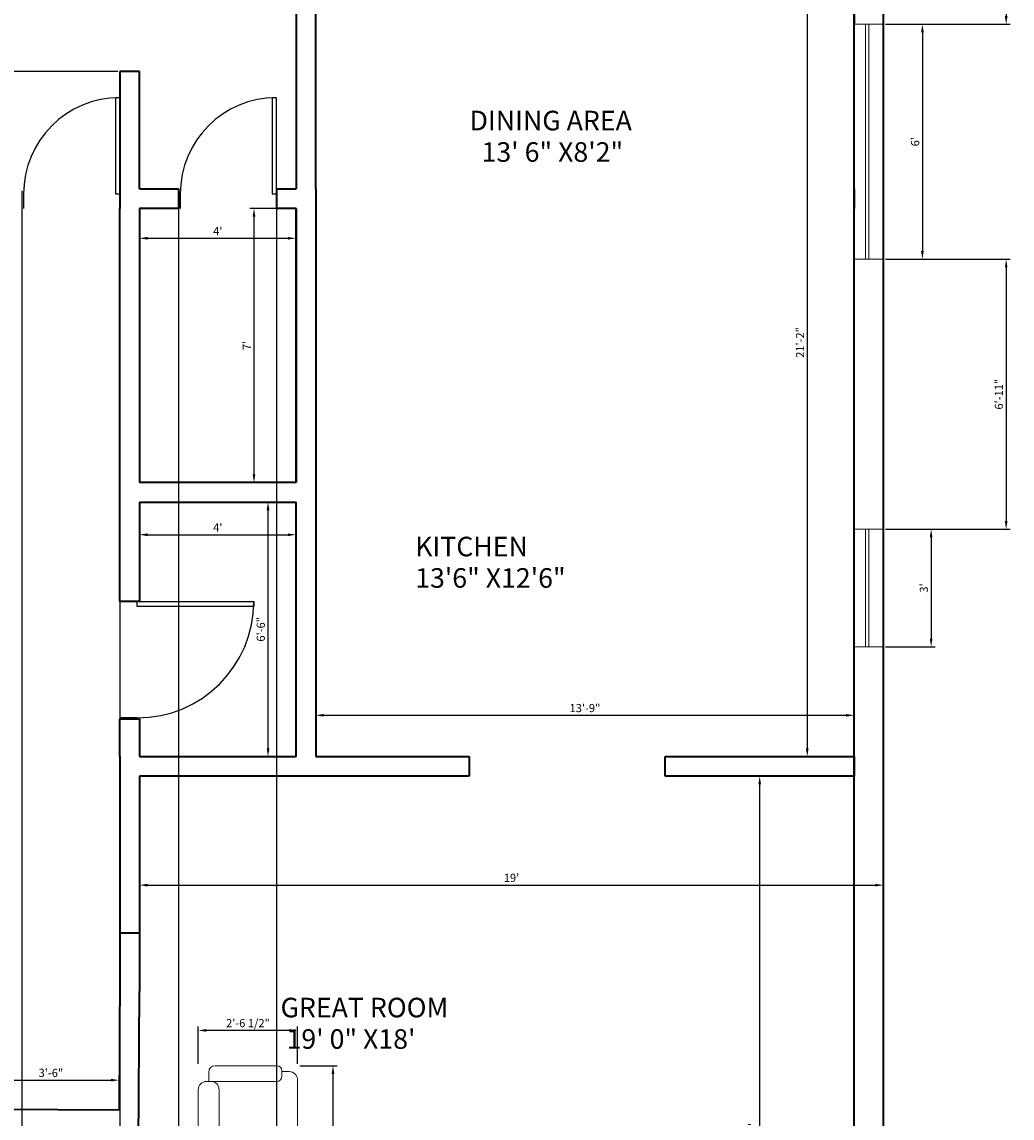
# Model space of a CAD drawing. Units: inches. Extents: x 2025 to 2528, y 1525 to 2336.
# Tile 8 of 18: x 2225 to 2528, y 1831 to 2167. Entities that reach past the tile are written whole.
import ezdxf

# ---------------------------------------------------------------- set-up
doc = ezdxf.new("R2010")
doc.units = ezdxf.units.IN
for name, color, linetype, lineweight in [('A-ANNO-DIMS', 2, 'Continuous', 18), ('A-AREA-IDEN', 7, 'Continuous', 25), ('A-DOOR', 3, 'Continuous', 25), ('A-FURN', 8, 'Continuous', 18), ('A-GLAZ', 4, 'Continuous', 18), ('A-WALL', 7, 'Continuous', 35)]:
    doc.layers.add(name, color=color, linetype=linetype, lineweight=lineweight)
doc.styles.get("Standard").update_dxf_attribs({"font": 'arial.ttf'})
doc.dimstyles.new('Copy of ISO-25', dxfattribs={"dimtxt": 2.5, "dimasz": 2.5, "dimexe": 1.25, "dimexo": 0.625, "dimtad": 1, "dimdec": 1, "dimlunit": 4, "dimtxsty": 'Standard', "dimcen": 2.5, "dimadec": 0, "dimazin": 0, "dimtfac": 1, "dimtdec": 1, "dimtmove": 0, "dimatfit": 3, "dimfxl": 1, "dimarcsym": 0})

# ---------------------------------------------------------------- blocks, each defined once
blk = doc.blocks.new('*U3')
for p, q in [((0, 0), (0, -6)), ((-40, 0), (-40, -6))]:
    blk.add_line(p, q)
blk.add_lwpolyline([(0, 0), (0, 40), (-1.75, 40), (-1.75, 0)], close=True)
blk.add_arc((0, 0), 40, 90, 180)
blk = doc.blocks.new('*U4')
for p, q in [((-40, 0), (-40, 6)), ((0, 0), (0, 6))]:
    blk.add_line(p, q)
blk.add_lwpolyline([(0, 0), (0, -40), (-1.75, -40), (-1.75, 0)], close=True)
blk.add_arc((0, 0), 40, 180, 270)
blk = doc.blocks.new('*D10')
at = {"layer": 'A-ANNO-DIMS', "color": 0, "lineweight": -2, "transparency": 16777216}
for p, q in [((2261.01, 2108.79), (2261.01, 2099)), ((2309.01, 2108.79), (2309.01, 2099)), ((2263.51, 2100.25), (2306.51, 2100.25))]:
    blk.add_line(p, q, dxfattribs=at)
at = {"layer": 'A-ANNO-DIMS', "color": 0, "transparency": 16777216}
for points in [[(2263.51, 2100.67), (2263.51, 2099.84), (2261.01, 2100.25)], [(2306.51, 2100.67), (2306.51, 2099.84), (2309.01, 2100.25)]]:
    blk.add_solid(points, dxfattribs=at)
at = {"layer": 'Defpoints', "color": 0, "transparency": 16777216}
for p in [(2261.01, 2109.41), (2309.01, 2109.41), (2309.01, 2100.25)]:
    blk.add_point(p, dxfattribs=at)
at = {"layer": 'A-ANNO-DIMS', "color": 0, "transparency": 16777216, "insert": (2285.01, 2102.13), "char_height": 2.5, "attachment_point": 5}
blk.add_mtext("4'", dxfattribs=at)
blk = doc.blocks.new('*D11')
at = {"layer": 'A-ANNO-DIMS', "color": 0, "lineweight": -2, "transparency": 16777216}
for p, q in [((2308.39, 2109.41), (2294.86, 2109.41)), ((2296.11, 2106.91), (2296.11, 2027.91)), ((2308.39, 2025.41), (2294.86, 2025.41))]:
    blk.add_line(p, q, dxfattribs=at)
at = {"layer": 'A-ANNO-DIMS', "color": 0, "transparency": 16777216}
for points in [[(2295.7, 2106.91), (2296.53, 2106.91), (2296.11, 2109.41)], [(2295.7, 2027.91), (2296.53, 2027.91), (2296.11, 2025.41)]]:
    blk.add_solid(points, dxfattribs=at)
at = {"layer": 'Defpoints', "color": 0, "transparency": 16777216}
for p in [(2309.01, 2109.41), (2296.11, 2025.41), (2309.01, 2025.41)]:
    blk.add_point(p, dxfattribs=at)
at = {"layer": 'A-ANNO-DIMS', "color": 0, "transparency": 16777216, "insert": (2294.24, 2067.41), "char_height": 2.5, "attachment_point": 5, "rotation": 90}
blk.add_mtext("7'", dxfattribs=at)
blk = doc.blocks.new('*D14')
at = {"layer": 'A-ANNO-DIMS', "color": 0, "lineweight": -2, "transparency": 16777216}
for p, q in [((2261.01, 2018.79), (2261.01, 2008.15)), ((2309.01, 2018.79), (2309.01, 2008.15)), ((2263.51, 2009.4), (2306.51, 2009.4))]:
    blk.add_line(p, q, dxfattribs=at)
at = {"layer": 'A-ANNO-DIMS', "color": 0, "transparency": 16777216}
for points in [[(2263.51, 2009.82), (2263.51, 2008.98), (2261.01, 2009.4)], [(2306.51, 2009.82), (2306.51, 2008.98), (2309.01, 2009.4)]]:
    blk.add_solid(points, dxfattribs=at)
at = {"layer": 'Defpoints', "color": 0, "transparency": 16777216}
for p in [(2261.01, 2019.41), (2309.01, 2019.41), (2309.01, 2009.4)]:
    blk.add_point(p, dxfattribs=at)
at = {"layer": 'A-ANNO-DIMS', "color": 0, "transparency": 16777216, "insert": (2285.01, 2011.27), "char_height": 2.5, "attachment_point": 5}
blk.add_mtext("4'", dxfattribs=at)
blk = doc.blocks.new('*D15')
at = {"layer": 'A-ANNO-DIMS', "color": 0, "lineweight": -2, "transparency": 16777216}
for p, q in [((2308.39, 2019.41), (2299.17, 2019.41)), ((2300.42, 1943.91), (2300.42, 2016.91)), ((2308.39, 1941.41), (2299.17, 1941.41))]:
    blk.add_line(p, q, dxfattribs=at)
at = {"layer": 'A-ANNO-DIMS', "color": 0, "transparency": 16777216}
for points in [[(2300.01, 2016.91), (2300.84, 2016.91), (2300.42, 2019.41)], [(2300.01, 1943.91), (2300.84, 1943.91), (2300.42, 1941.41)]]:
    blk.add_solid(points, dxfattribs=at)
at = {"layer": 'Defpoints', "color": 0, "transparency": 16777216}
for p in [(2300.42, 2019.41), (2309.01, 2019.41), (2309.01, 1941.41)]:
    blk.add_point(p, dxfattribs=at)
at = {"layer": 'A-ANNO-DIMS', "color": 0, "transparency": 16777216, "insert": (2298.52, 1980.41), "char_height": 2.5, "attachment_point": 5, "rotation": 90}
blk.add_mtext('6\'-6"', dxfattribs=at)
blk = doc.blocks.new('*D18')
at = {"layer": 'A-ANNO-DIMS', "color": 0, "lineweight": -2, "transparency": 16777216}
for p, q in [((2479.39, 2195.22), (2464.37, 2195.22)), ((2465.62, 2192.72), (2465.62, 1943.91)), ((2479.39, 1941.41), (2464.37, 1941.41))]:
    blk.add_line(p, q, dxfattribs=at)
at = {"layer": 'A-ANNO-DIMS', "color": 0, "transparency": 16777216}
for points in [[(2465.2, 2192.72), (2466.03, 2192.72), (2465.62, 2195.22)], [(2465.2, 1943.91), (2466.03, 1943.91), (2465.62, 1941.41)]]:
    blk.add_solid(points, dxfattribs=at)
at = {"layer": 'Defpoints', "color": 0, "transparency": 16777216}
for p in [(2480.01, 2195.22), (2465.62, 1941.41), (2480.01, 1941.41)]:
    blk.add_point(p, dxfattribs=at)
at = {"layer": 'A-ANNO-DIMS', "color": 0, "transparency": 16777216, "insert": (2463.74, 2068.31), "char_height": 2.5, "attachment_point": 5, "rotation": 90}
blk.add_mtext('21\'-2"', dxfattribs=at)
blk = doc.blocks.new('*D19')
at = {"layer": 'A-ANNO-DIMS', "color": 0, "lineweight": -2, "transparency": 16777216}
for p, q in [((2315.01, 1942.04), (2315.01, 1955.31)), ((2480.01, 1942.04), (2480.01, 1955.31)), ((2317.51, 1954.06), (2477.51, 1954.06))]:
    blk.add_line(p, q, dxfattribs=at)
at = {"layer": 'A-ANNO-DIMS', "color": 0, "transparency": 16777216}
for points in [[(2317.51, 1954.48), (2317.51, 1953.64), (2315.01, 1954.06)], [(2477.51, 1954.48), (2477.51, 1953.64), (2480.01, 1954.06)]]:
    blk.add_solid(points, dxfattribs=at)
at = {"layer": 'Defpoints', "color": 0, "transparency": 16777216}
for p in [(2480.01, 1954.06), (2315.01, 1941.41), (2480.01, 1941.41)]:
    blk.add_point(p, dxfattribs=at)
at = {"layer": 'A-ANNO-DIMS', "color": 0, "transparency": 16777216, "insert": (2397.51, 1955.96), "char_height": 2.5, "attachment_point": 5}
blk.add_mtext('13\'-9"', dxfattribs=at)
blk = doc.blocks.new('*D23')
at = {"layer": 'A-ANNO-DIMS', "color": 0, "lineweight": -2, "transparency": 16777216}
for p, q in [((2489.64, 2011.08), (2504.83, 2011.08)), ((2503.58, 2008.58), (2503.58, 1977.58)), ((2489.64, 1975.08), (2504.83, 1975.08))]:
    blk.add_line(p, q, dxfattribs=at)
at = {"layer": 'A-ANNO-DIMS', "color": 0, "transparency": 16777216}
for points in [[(2503.16, 2008.58), (2504, 2008.58), (2503.58, 2011.08)], [(2503.16, 1977.58), (2504, 1977.58), (2503.58, 1975.08)]]:
    blk.add_solid(points, dxfattribs=at)
at = {"layer": 'Defpoints', "color": 0, "transparency": 16777216}
for p in [(2489.01, 2011.08), (2489.01, 1975.08), (2503.58, 1975.08)]:
    blk.add_point(p, dxfattribs=at)
at = {"layer": 'A-ANNO-DIMS', "color": 0, "transparency": 16777216, "insert": (2501.68, 1993.08), "char_height": 2.5, "attachment_point": 5, "rotation": 90}
blk.add_mtext("3'", dxfattribs=at)
blk = doc.blocks.new('*D24')
at = {"layer": 'A-ANNO-DIMS', "color": 0, "lineweight": -2, "transparency": 16777216}
for p, q in [((2489.64, 2165.84), (2502.15, 2165.84)), ((2500.9, 2163.34), (2500.9, 2096.34)), ((2489.64, 2093.84), (2502.15, 2093.84))]:
    blk.add_line(p, q, dxfattribs=at)
at = {"layer": 'A-ANNO-DIMS', "color": 0, "transparency": 16777216}
for points in [[(2500.48, 2163.34), (2501.32, 2163.34), (2500.9, 2165.84)], [(2500.48, 2096.34), (2501.32, 2096.34), (2500.9, 2093.84)]]:
    blk.add_solid(points, dxfattribs=at)
at = {"layer": 'Defpoints', "color": 0, "transparency": 16777216}
for p in [(2489.01, 2165.84), (2489.01, 2093.84), (2500.9, 2093.84)]:
    blk.add_point(p, dxfattribs=at)
at = {"layer": 'A-ANNO-DIMS', "color": 0, "transparency": 16777216, "insert": (2499, 2129.84), "char_height": 2.5, "attachment_point": 5, "rotation": 90}
blk.add_mtext("6'", dxfattribs=at)
blk = doc.blocks.new('*D31')
at = {"layer": 'A-ANNO-DIMS', "color": 0, "lineweight": -2, "transparency": 16777216}
for p, q in [((2479.39, 1935.41), (2449.8, 1935.41)), ((2451.05, 1715.91), (2451.05, 1932.91)), ((2479.39, 1713.41), (2449.8, 1713.41))]:
    blk.add_line(p, q, dxfattribs=at)
at = {"layer": 'A-ANNO-DIMS', "color": 0, "transparency": 16777216}
for points in [[(2450.63, 1932.91), (2451.46, 1932.91), (2451.05, 1935.41)], [(2450.63, 1715.91), (2451.46, 1715.91), (2451.05, 1713.41)]]:
    blk.add_solid(points, dxfattribs=at)
at = {"layer": 'Defpoints', "color": 0, "transparency": 16777216}
for p in [(2451.05, 1935.41), (2480.01, 1935.41), (2480.01, 1713.41)]:
    blk.add_point(p, dxfattribs=at)
at = {"layer": 'A-ANNO-DIMS', "color": 0, "transparency": 16777216, "insert": (2449.15, 1824.41), "char_height": 2.5, "attachment_point": 5, "rotation": 90}
blk.add_mtext('18\'-6"', dxfattribs=at)
blk = doc.blocks.new('*D32')
at = {"layer": 'A-ANNO-DIMS', "color": 0, "lineweight": -2, "transparency": 16777216}
for p, q in [((2261.01, 1934.79), (2261.01, 1900.76)), ((2489.01, 1934.79), (2489.01, 1900.76)), ((2263.51, 1902.01), (2486.51, 1902.01))]:
    blk.add_line(p, q, dxfattribs=at)
at = {"layer": 'A-ANNO-DIMS', "color": 0, "transparency": 16777216}
for points in [[(2263.51, 1902.42), (2263.51, 1901.59), (2261.01, 1902.01)], [(2486.51, 1902.42), (2486.51, 1901.59), (2489.01, 1902.01)]]:
    blk.add_solid(points, dxfattribs=at)
at = {"layer": 'Defpoints', "color": 0, "transparency": 16777216}
for p in [(2261.01, 1935.41), (2489.01, 1935.41), (2489.01, 1902.01)]:
    blk.add_point(p, dxfattribs=at)
at = {"layer": 'A-ANNO-DIMS', "color": 0, "transparency": 16777216, "insert": (2375.01, 1903.91), "char_height": 2.5, "attachment_point": 5}
blk.add_mtext("19'", dxfattribs=at)
blk = doc.blocks.new('*D35')
at = {"layer": 'A-ANNO-DIMS', "color": 0, "lineweight": -2, "transparency": 16777216}
for p, q in [((2213.01, 1834.04), (2213.01, 1843.49)), ((2215.51, 1842.24), (2252.28, 1842.24)), ((2254.78, 1833.8), (2254.78, 1843.49))]:
    blk.add_line(p, q, dxfattribs=at)
at = {"layer": 'A-ANNO-DIMS', "color": 0, "transparency": 16777216}
for points in [[(2215.51, 1842.66), (2215.51, 1841.83), (2213.01, 1842.24)], [(2252.28, 1842.66), (2252.28, 1841.83), (2254.78, 1842.24)]]:
    blk.add_solid(points, dxfattribs=at)
at = {"layer": 'Defpoints', "color": 0, "transparency": 16777216}
for p in [(2254.78, 1842.24), (2213.01, 1833.41), (2254.78, 1833.18)]:
    blk.add_point(p, dxfattribs=at)
at = {"layer": 'A-ANNO-DIMS', "color": 0, "transparency": 16777216, "insert": (2233.89, 1844.15), "char_height": 2.5, "attachment_point": 5}
blk.add_mtext('3\'-6"', dxfattribs=at)
blk = doc.blocks.new('A$C0876780F')
for p, q in [((0.72, 0.95), (0.23, 0.95)), ((1.32, 0.95), (0.88, 0.95)), ((1.48, 0.95), (2.02, 0.95)), ((0.15, 0.85), (0.06, 0.85)), ((0.15, 0.87), (0.15, 0.844)), ((0.15, 0.87), (0.15, 0.85)), ((0.15, 0.21), (0.15, 0.85)), ((0.8, 0.85), (0.8, 0.87)), ((0.8, 0.87), (0.8, 0.85)), ((0.8, 0.87), (0.8, 0.844)), ((1.4, 0.85), (1.4, 0.87)), ((1.4, 0.85), (1.4, 0.87)), ((2.1, 0.87), (2.1, 0.85)), ((2.1, 0.87), (2.1, 0.844)), ((2.1, 0.21), (2.1, 0.85)), ((2.1, 0.85), (2.19, 0.85)), ((0, 0.79), (0, 0.21)), ((0.72, 0.75), (0.23, 0.75)), ((0.801, 0.82), (0.801, 0.08)), ((1.32, 0.75), (0.88, 0.75)), ((1.401, 0.08), (1.401, 0.803)), ((1.48, 0.75), (2.02, 0.75)), ((2.25, 0.79), (2.25, 0.21)), ((0, 0.21), (0, 0.2)), ((0.15, 0.2), (0.15, 0.25)), ((2.1, 0.2), (2.1, 0.25)), ((2.25, 0.21), (2.25, 0.2)), ((0.05, 0.15), (0.1, 0.15)), ((0.056, 0.15), (0.056, 0.08)), ((2.2, 0.15), (2.15, 0.15)), ((2.194, 0.15), (2.194, 0.08)), ((0.136, 0), (0.709, 0)), ((0.801, 0.07), (0.801, 0.08)), ((0.871, 0), (1.331, 0)), ((1.401, 0.07), (1.401, 0.08)), ((2.114, 0), (1.48, 0))]:
    blk.add_line(p, q)
for centre, radius, start, end in [((0.23, 0.87), 0.08, 90, 180), ((0.72, 0.87), 0.08, 0, 90), ((0.88, 0.87), 0.08, 90, 180), ((1.32, 0.87), 0.08, 0, 90), ((1.48, 0.87), 0.08, 90, 180), ((2.02, 0.87), 0.08, 0, 90), ((0.06, 0.79), 0.06, 90, 180), ((2.19, 0.79), 0.06, 0, 90), ((0.23, 0.83), 0.08, 180, 270), ((0.23, 0.83), 0.08, 180, 270), ((0.72, 0.83), 0.08, 270, 0), ((0.88, 0.83), 0.08, 180, 270), ((0.88, 0.83), 0.08, 180, 270), ((1.32, 0.83), 0.08, 270, 0), ((1.48, 0.83), 0.08, 180, 270), ((2.02, 0.83), 0.08, 270, 0), ((2.02, 0.83), 0.08, 270, 0), ((0.09, 0.21), 0.06, 350.5377, 0), ((2.16, 0.21), 0.06, 180, 189.4623), ((0.05, 0.2), 0.05, 180, 270), ((0.1, 0.2), 0.05, 270, 0), ((2.15, 0.2), 0.05, 180, 270), ((2.2, 0.2), 0.05, 270, 0), ((0.136, 0.08), 0.08, 180, 270), ((0.721, 0.08), 0.08, 270, 0), ((0.871, 0.07), 0.07, 180, 270), ((1.331, 0.07), 0.07, 270, 0), ((1.481, 0.08), 0.08, 180, 270), ((2.114, 0.08), 0.08, 270, 0)]:
    blk.add_arc(centre, radius, start, end)
blk = doc.blocks.new('WIN-36-EXT')
for p, q in [((0, 0), (0, 9)), ((0, 9), (36, 9)), ((36, 9), (36, 0)), ((0, 4.5), (36, 4.5)), ((0, 3.5), (36, 3.5))]:
    blk.add_line(p, q)
blk = doc.blocks.new('*D58')
at = {"layer": 'A-ANNO-DIMS', "color": 0, "lineweight": -2, "transparency": 16777216}
for p, q in [((2310.12, 1846.66), (2321.57, 1846.66)), ((2320.32, 1777.01), (2320.32, 1844.16)), ((2310.12, 1774.51), (2321.57, 1774.51))]:
    blk.add_line(p, q, dxfattribs=at)
at = {"layer": 'A-ANNO-DIMS', "color": 0, "transparency": 16777216}
for points in [[(2319.9, 1844.16), (2320.73, 1844.16), (2320.32, 1846.66)], [(2319.9, 1777.01), (2320.73, 1777.01), (2320.32, 1774.51)]]:
    blk.add_solid(points, dxfattribs=at)
at = {"layer": 'Defpoints', "color": 0, "transparency": 16777216}
for p in [(2309.49, 1846.66), (2320.32, 1846.66), (2309.49, 1774.51)]:
    blk.add_point(p, dxfattribs=at)
at = {"layer": 'A-ANNO-DIMS', "color": 0, "transparency": 16777216, "insert": (2318.4, 1810.58), "char_height": 2.5, "attachment_point": 5, "rotation": 90}
blk.add_mtext('SOFA 6\'-0"', dxfattribs=at)
blk = doc.blocks.new('*D59')
at = {"layer": 'A-ANNO-DIMS', "color": 0, "lineweight": -2, "transparency": 16777216}
for p, q in [((2279.03, 1847.29), (2279.03, 1858.73)), ((2309.49, 1847.29), (2309.49, 1858.73)), ((2306.99, 1857.48), (2281.53, 1857.48))]:
    blk.add_line(p, q, dxfattribs=at)
at = {"layer": 'A-ANNO-DIMS', "color": 0, "transparency": 16777216}
for points in [[(2281.53, 1857.9), (2281.53, 1857.07), (2279.03, 1857.48)], [(2306.99, 1857.9), (2306.99, 1857.07), (2309.49, 1857.48)]]:
    blk.add_solid(points, dxfattribs=at)
at = {"layer": 'Defpoints', "color": 0, "transparency": 16777216}
for p in [(2279.03, 1857.48), (2279.03, 1846.66), (2309.49, 1846.66)]:
    blk.add_point(p, dxfattribs=at)
at = {"layer": 'A-ANNO-DIMS', "color": 0, "transparency": 16777216, "insert": (2294.26, 1859.4), "char_height": 2.5, "attachment_point": 5}
blk.add_mtext('2\'-6 1/2"', dxfattribs=at)
blk = doc.blocks.new('*D63')
at = {"layer": 'A-ANNO-DIMS', "color": 0, "lineweight": -2, "transparency": 16777216}
for p, q in [((2489.64, 2292.41), (2527.81, 2292.41)), ((2526.56, 2289.91), (2526.56, 2168.34)), ((2489.64, 2165.84), (2527.81, 2165.84))]:
    blk.add_line(p, q, dxfattribs=at)
at = {"layer": 'A-ANNO-DIMS', "color": 0, "transparency": 16777216}
for points in [[(2526.15, 2289.91), (2526.98, 2289.91), (2526.56, 2292.41)], [(2526.15, 2168.34), (2526.98, 2168.34), (2526.56, 2165.84)]]:
    blk.add_solid(points, dxfattribs=at)
at = {"layer": 'Defpoints', "color": 0, "transparency": 16777216}
for p in [(2489.01, 2292.41), (2489.01, 2165.84), (2526.56, 2165.84)]:
    blk.add_point(p, dxfattribs=at)
at = {"layer": 'A-ANNO-DIMS', "color": 0, "transparency": 16777216, "insert": (2524.65, 2229.13), "char_height": 2.5, "attachment_point": 5, "rotation": 90}
blk.add_mtext('10\'-6 1/2"', dxfattribs=at)
blk = doc.blocks.new('*D64')
at = {"layer": 'A-ANNO-DIMS', "color": 0, "lineweight": -2, "transparency": 16777216}
for p, q in [((2489.64, 2093.84), (2527.81, 2093.84)), ((2526.56, 2091.34), (2526.56, 2013.58)), ((2489.64, 2011.08), (2527.81, 2011.08))]:
    blk.add_line(p, q, dxfattribs=at)
at = {"layer": 'A-ANNO-DIMS', "color": 0, "transparency": 16777216}
for points in [[(2526.15, 2091.34), (2526.98, 2091.34), (2526.56, 2093.84)], [(2526.15, 2013.58), (2526.98, 2013.58), (2526.56, 2011.08)]]:
    blk.add_solid(points, dxfattribs=at)
at = {"layer": 'Defpoints', "color": 0, "transparency": 16777216}
for p in [(2489.01, 2093.84), (2489.01, 2011.08), (2526.56, 2011.08)]:
    blk.add_point(p, dxfattribs=at)
at = {"layer": 'A-ANNO-DIMS', "color": 0, "transparency": 16777216, "insert": (2524.66, 2052.46), "char_height": 2.5, "attachment_point": 5, "rotation": 90}
blk.add_mtext('6\'-11"', dxfattribs=at)
blk = doc.blocks.new('*D75')
at = {"layer": 'A-ANNO-DIMS', "color": 0, "lineweight": -2, "transparency": 16777216}
for p, q in [((2225.01, 2114.79), (2225.01, 1525.61)), ((2255.01, 2114.79), (2255.01, 1525.61)), ((2227.51, 1526.86), (2252.51, 1526.86))]:
    blk.add_line(p, q, dxfattribs=at)
at = {"layer": 'A-ANNO-DIMS', "color": 0, "transparency": 16777216}
for points in [[(2227.51, 1527.28), (2227.51, 1526.45), (2225.01, 1526.86)], [(2252.51, 1527.28), (2252.51, 1526.45), (2255.01, 1526.86)]]:
    blk.add_solid(points, dxfattribs=at)
at = {"layer": 'Defpoints', "color": 0, "transparency": 16777216}
for p in [(2225.01, 2115.41), (2255.01, 2115.41), (2255.01, 1526.86)]:
    blk.add_point(p, dxfattribs=at)
at = {"layer": 'A-ANNO-DIMS', "color": 0, "transparency": 16777216, "insert": (2240.01, 1528.76), "char_height": 2.5, "attachment_point": 5}
blk.add_mtext('2\'-6"', dxfattribs=at)
blk = doc.blocks.new('*D76')
at = {"layer": 'A-ANNO-DIMS', "color": 0, "lineweight": -2, "transparency": 16777216}
for p, q in [((2273.01, 2114.79), (2273.01, 1525.61)), ((2303.01, 2114.79), (2303.01, 1525.61)), ((2275.51, 1526.86), (2300.51, 1526.86))]:
    blk.add_line(p, q, dxfattribs=at)
at = {"layer": 'A-ANNO-DIMS', "color": 0, "transparency": 16777216}
for points in [[(2275.51, 1527.28), (2275.51, 1526.45), (2273.01, 1526.86)], [(2300.51, 1527.28), (2300.51, 1526.45), (2303.01, 1526.86)]]:
    blk.add_solid(points, dxfattribs=at)
at = {"layer": 'Defpoints', "color": 0, "transparency": 16777216}
for p in [(2273.01, 2115.41), (2303.01, 2115.41), (2303.01, 1526.86)]:
    blk.add_point(p, dxfattribs=at)
at = {"layer": 'A-ANNO-DIMS', "color": 0, "transparency": 16777216, "insert": (2288.01, 1528.76), "char_height": 2.5, "attachment_point": 5}
blk.add_mtext('2\'-6"', dxfattribs=at)
blk = doc.blocks.new('*D77')
at = {"layer": 'A-ANNO-DIMS', "color": 0, "lineweight": -2, "transparency": 16777216}
for p, q in [((2254.39, 2181.41), (2027.21, 2181.41)), ((2028.46, 2153.91), (2028.46, 2178.91)), ((2254.39, 2151.41), (2027.21, 2151.41))]:
    blk.add_line(p, q, dxfattribs=at)
at = {"layer": 'A-ANNO-DIMS', "color": 0, "transparency": 16777216}
for points in [[(2028.05, 2178.91), (2028.88, 2178.91), (2028.46, 2181.41)], [(2028.05, 2153.91), (2028.88, 2153.91), (2028.46, 2151.41)]]:
    blk.add_solid(points, dxfattribs=at)
at = {"layer": 'Defpoints', "color": 0, "transparency": 16777216}
for p in [(2028.46, 2181.41), (2255.01, 2181.41), (2255.01, 2151.41)]:
    blk.add_point(p, dxfattribs=at)
at = {"layer": 'A-ANNO-DIMS', "color": 0, "transparency": 16777216, "insert": (2026.56, 2166.41), "char_height": 2.5, "attachment_point": 5, "rotation": 90}
blk.add_mtext('2\'-6"', dxfattribs=at)
blk = doc.blocks.new('*D80')
at = {"layer": 'A-ANNO-DIMS', "color": 0, "lineweight": -2, "transparency": 16777216}
for p, q in [((2065.39, 2292.41), (2027.21, 2292.41)), ((2028.46, 1566.91), (2028.46, 2289.91)), ((2285.39, 1564.41), (2027.21, 1564.41))]:
    blk.add_line(p, q, dxfattribs=at)
at = {"layer": 'A-ANNO-DIMS', "color": 0, "transparency": 16777216}
for points in [[(2028.05, 2289.91), (2028.88, 2289.91), (2028.46, 2292.41)], [(2028.05, 1566.91), (2028.88, 1566.91), (2028.46, 1564.41)]]:
    blk.add_solid(points, dxfattribs=at)
at = {"layer": 'Defpoints', "color": 0, "transparency": 16777216}
for p in [(2028.46, 2292.41), (2066.01, 2292.41), (2286.01, 1564.41)]:
    blk.add_point(p, dxfattribs=at)
at = {"layer": 'A-ANNO-DIMS', "color": 0, "transparency": 16777216, "insert": (2026.56, 1928.41), "char_height": 2.5, "attachment_point": 5, "rotation": 90}
blk.add_mtext('60\'-8"', dxfattribs=at)

msp = doc.modelspace()

# ---------------------------------------------------------------- linework, layer by layer
at = {"layer": 'A-GLAZ'}
for p, q in [((2480.01, 2165.84), (2489.01, 2165.84)), ((2483.51, 2165.84), (2483.51, 2093.84)), ((2484.51, 2165.84), (2484.51, 2093.84)), ((2489.01, 2165.84), (2489.01, 2093.84)), ((2489.01, 2165.84), (2489.01, 2093.84)), ((2489.01, 2093.84), (2480.01, 2093.84)), ((2489.01, 2011.08), (2489.01, 2011.08))]:
    msp.add_line(p, q, dxfattribs=at)
at = {"layer": 'A-WALL'}
for p, q in [((2309.01, 2283.41), (2309.01, 2115.41)), ((2315.01, 2115.41), (2315.01, 2283.41)), ((2489.01, 1704.41), (2489.01, 2283.41)), ((2480.01, 1713.41), (2480.01, 2195.22)), ((2480.01, 2195.22), (2480.01, 2165.84)), ((2261.01, 2151.41), (2255.01, 2151.41)), ((2255.01, 2151.41), (2255.01, 2115.41)), ((2261.01, 2115.41), (2261.01, 2151.41)), ((2255.01, 2115.41), (2255.01, 2109.41)), ((2261.01, 2115.41), (2261.01, 2115.41)), ((2261.01, 2115.41), (2273.01, 2115.41)), ((2261.01, 2115.41), (2273.01, 2115.41)), ((2273.01, 2115.41), (2273.01, 2109.41)), ((2303.01, 2115.41), (2303.01, 2109.41)), ((2303.01, 2115.41), (2309.01, 2115.41)), ((2315.01, 2115.41), (2315.01, 2109.41)), ((2480.01, 2115.41), (2480.01, 2109.41)), ((2255.01, 1988.95), (2255.01, 2109.41)), ((2261.01, 2109.41), (2261.01, 2025.41)), ((2273.01, 2109.41), (2261.01, 2109.41)), ((2309.01, 2109.41), (2303.01, 2109.41)), ((2309.01, 2109.41), (2309.01, 2025.41)), ((2309.01, 2025.41), (2309.01, 2109.41)), ((2315.01, 2109.41), (2315.01, 1941.41)), ((2309.01, 2025.41), (2261.01, 2025.41)), ((2261.01, 2019.41), (2309.01, 2019.41)), ((2261.01, 2019.41), (2261.01, 1988.95)), ((2309.01, 1941.41), (2309.01, 2019.41)), ((2261.01, 1988.95), (2255.01, 1988.95)), ((2480.01, 1941.41), (2480.01, 1975.08)), ((2255.01, 1941.41), (2255.01, 1952.95)), ((2255.01, 1941.41), (2255.01, 1952.95)), ((2255.01, 1952.95), (2261.01, 1952.95)), ((2261.01, 1952.95), (2261.01, 1941.41)), ((2255.01, 1941.41), (2255.01, 1941.41)), ((2255.01, 1941.41), (2255.01, 1875.41)), ((2261.01, 1941.41), (2309.01, 1941.41)), ((2315.01, 1941.41), (2362.08, 1941.41)), ((2315.01, 1941.41), (2362.08, 1941.41)), ((2362.08, 1941.41), (2362.08, 1935.41)), ((2422.08, 1935.41), (2422.08, 1941.41)), ((2422.08, 1941.41), (2480.01, 1941.41)), ((2480.01, 1941.41), (2480.01, 1935.41)), ((2261.01, 1935.41), (2261.01, 1875.41)), ((2309.01, 1935.41), (2261.01, 1935.41)), ((2315.01, 1935.41), (2309.01, 1935.41)), ((2362.08, 1935.41), (2315.01, 1935.41)), ((2480.01, 1935.41), (2422.08, 1935.41)), ((2255.01, 1887.41), (2261.01, 1887.41)), ((2255.01, 1875.41), (2254.78, 1833.18)), ((2261.01, 1875.41), (2261.01, 1869.41)), ((2260.29, 1744.82), (2261.01, 1869.41)), ((2213.01, 1833.41), (2254.78, 1833.18))]:
    msp.add_line(p, q, dxfattribs=at)

# ---------------------------------------------------------------- block references
at = {"layer": 'A-DOOR', "xscale": 0.7375996643662327, "yscale": 0.7375996643662327, "zscale": 0.7375996643662327}
for p in [(2255.01, 2113.84), (2303.01, 2113.84)]:
    msp.add_blockref('*U3', p, dxfattribs=at)
at = {"layer": 'A-DOOR', "xscale": 0.8923728301010077, "yscale": 0.8923728301010077, "zscale": 0.8923728301010077, "rotation": 90}
msp.add_blockref('*U4', (2260.37, 1988.95), dxfattribs=at)
at = {"layer": 'A-FURN', "xscale": 32.06799314308715, "yscale": 32.06799314308715, "zscale": 32.06799314308715, "rotation": 90}
msp.add_blockref('A$C0876780F', (2309.49, 1774.51), dxfattribs=at)
at = {"layer": 'A-GLAZ', "rotation": 270.0000000000033}
msp.add_blockref('WIN-36-EXT', (2480.01, 2011.08), dxfattribs=at)

# ---------------------------------------------------------------- texts
at = {"layer": 'A-AREA-IDEN'}
for s, p in [('DINING AREA', (2362.17, 2133.33)), ('  13\' 6" X8\'2"', (2362.17, 2123.69)), ('KITCHEN', (2345.5, 2002.78)), ('13\'6" X12\'6"', (2345.5, 1993.15)), ('GREAT ROOM', (2304.25, 1861.49)), (' 19\' 0" X18\'', (2304.25, 1851.85))]:
    msp.add_text(s, height=6, dxfattribs=at).set_placement(p)

# ---------------------------------------------------------------- dimensions: what is measured, and where the dimension line sits
at = {"layer": 'A-ANNO-DIMS'}
for base, p1, p2, angle, override, picture, middle in [((2028.46, 2292.41), (2286.01, 1564.41), (2066.01, 2292.41), 90, {"dimdec": 1, "dimlfac": 1, "dimrnd": 0, "dimzin": 1, "dimdsep": 46, "dimlunit": 4, "dimfrac": 2}, '*D80', (2026.56, 1928.41)), ((2526.56, 2165.84), (2489.01, 2292.41), (2489.01, 2165.84), 90, {"dimdec": 1, "dimlfac": 1, "dimrnd": 0, "dimzin": 1, "dimdsep": 46, "dimlunit": 4, "dimfrac": 2}, '*D63', (2524.65, 2229.13)), ((2465.62, 1941.41), (2480.01, 2195.22), (2480.01, 1941.41), 90, {"dimclrd": 0, "dimclre": 0, "dimclrt": 0}, '*D18', (2463.74, 2068.31)), ((2028.46, 2181.41), (2255.01, 2151.41), (2255.01, 2181.41), 90, {"dimdec": 1, "dimlfac": 1, "dimrnd": 0, "dimzin": 1, "dimdsep": 46, "dimlunit": 4, "dimfrac": 2}, '*D77', (2026.56, 2166.41)), ((2500.9, 2093.84), (2489.01, 2165.84), (2489.01, 2093.84), 90, {"dimclrd": 0, "dimclre": 0, "dimclrt": 0}, '*D24', (2499, 2129.84)), ((2296.11, 2025.41), (2309.01, 2109.41), (2309.01, 2025.41), 90, {"dimclrd": 0, "dimclre": 0, "dimclrt": 0}, '*D11', (2294.24, 2067.41)), ((2526.56, 2011.08), (2489.01, 2093.84), (2489.01, 2011.08), 90, {"dimdec": 1, "dimlfac": 1, "dimrnd": 0, "dimzin": 1, "dimdsep": 46, "dimlunit": 4, "dimfrac": 2}, '*D64', (2524.66, 2052.46)), ((2300.42, 2019.41), (2309.01, 1941.41), (2309.01, 2019.41), 90, {"dimclrd": 0, "dimclre": 0, "dimclrt": 0}, '*D15', (2298.52, 1980.41)), ((2503.58, 1975.08), (2489.01, 2011.08), (2489.01, 1975.08), 90, {"dimclrd": 0, "dimclre": 0, "dimclrt": 0}, '*D23', (2501.68, 1993.08)), ((2451.05, 1935.41), (2480.01, 1713.41), (2480.01, 1935.41), 90, {"dimclrd": 0, "dimclre": 0, "dimclrt": 0}, '*D31', (2449.15, 1824.41)), ((2279.03, 1857.48), (2309.49, 1846.66), (2279.03, 1846.66), 180, {"dimdec": 1, "dimlfac": 1, "dimrnd": 0, "dimzin": 1, "dimdsep": 46, "dimlunit": 4, "dimfrac": 2}, '*D59', (2294.26, 1859.4))]:
    dim = msp.add_linear_dim(base=base, p1=p1, p2=p2, angle=angle, dimstyle='Copy of ISO-25', override=override, dxfattribs=at)
    dim.commit()
    dim.dimension.update_dxf_attribs({"geometry": picture, "text_midpoint": middle})
for base, p1, p2, override, picture, middle in [((2255.01, 1526.86), (2225.01, 2115.41), (2255.01, 2115.41), {"dimdec": 1, "dimlfac": 1, "dimrnd": 0, "dimzin": 1, "dimdsep": 46, "dimlunit": 4, "dimfrac": 2}, '*D75', (2240.01, 1528.76)), ((2303.01, 1526.86), (2273.01, 2115.41), (2303.01, 2115.41), {"dimdec": 1, "dimlfac": 1, "dimrnd": 0, "dimzin": 1, "dimdsep": 46, "dimlunit": 4, "dimfrac": 2}, '*D76', (2288.01, 1528.76)), ((2309.01, 2100.25), (2261.01, 2109.41), (2309.01, 2109.41), {"dimclrd": 0, "dimclre": 0, "dimclrt": 0}, '*D10', (2285.01, 2102.13)), ((2309.01, 2009.4), (2261.01, 2019.41), (2309.01, 2019.41), {"dimclrd": 0, "dimclre": 0, "dimclrt": 0}, '*D14', (2285.01, 2011.27)), ((2480.01, 1954.06), (2315.01, 1941.41), (2480.01, 1941.41), {"dimclrd": 0, "dimclre": 0, "dimclrt": 0}, '*D19', (2397.51, 1955.96)), ((2489.01, 1902.01), (2261.01, 1935.41), (2489.01, 1935.41), {"dimclrd": 0, "dimclre": 0, "dimclrt": 0}, '*D32', (2375.01, 1903.91)), ((2254.78, 1842.24), (2213.01, 1833.41), (2254.78, 1833.18), {"dimclrd": 0, "dimclre": 0, "dimclrt": 0}, '*D35', (2233.89, 1844.15))]:
    dim = msp.add_linear_dim(base=base, p1=p1, p2=p2, dimstyle='Copy of ISO-25', override=override, dxfattribs=at)
    dim.commit()
    dim.dimension.update_dxf_attribs({"geometry": picture, "text_midpoint": middle})
dim = msp.add_linear_dim(base=(2320.3169, 1846.6606), p1=(2309.494, 1774.5076), p2=(2309.494, 1846.6606), angle=90, text='SOFA <>', dimstyle='Copy of ISO-25', override={"dimdec": 1, "dimlfac": 1, "dimrnd": 0, "dimzin": 1, "dimdsep": 46, "dimlunit": 4, "dimfrac": 2}, dxfattribs=at)
dim.commit()
dim.dimension.update_dxf_attribs({"geometry": '*D58', "text_midpoint": (2318.3984, 1810.5841)})

doc.saveas('drawing.dxf')
